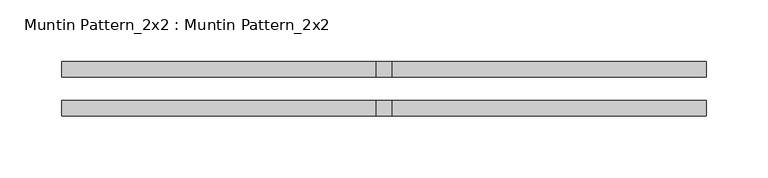
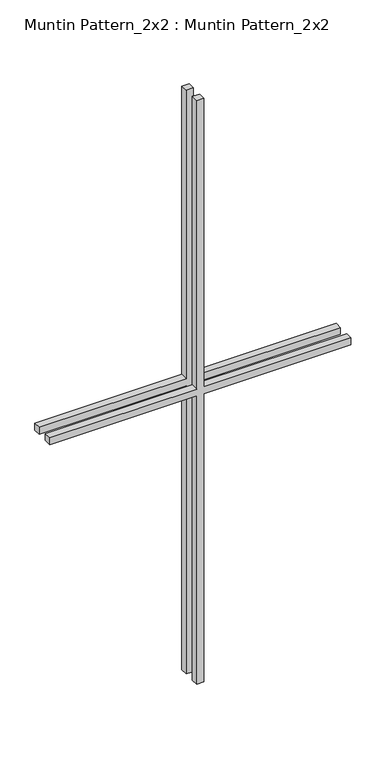
"""IFC4 building model written with IfcOpenShell, lengths in millimetres: proxy geometry, Muntin Pattern_2x2 : Muntin Pattern_2x2."""

from ifc_helpers import new_model, si_unit, frame, origin, place, context, project, spatial, polyline, outline, extrude, source, transform, mapped, element, save


def muntin_pattern_2x2_muntin_pattern_2x2_c2d27229(model_context):
    return source(origin(), model_context, "Body", "SweptSolid", [
        extrude(outline(polyline([(542.925, -6.35), (542.925, -261.9375), (530.225, -261.9375), (530.225, -6.35), (0.0, -6.35), (0.0, 6.35), (530.225, 6.35), (530.225, 261.9375), (542.925, 261.9375), (542.925, 6.35), (1073.15, 6.35), (1073.15, -6.35), (542.925, -6.35)])), frame((0.0, -22.225, 0.0), z_axis=(0.0, 1.0, 0.0), x_axis=(0.0, 0.0, 1.0)), (0.0, 0.0, 1.0), 12.7),
        extrude(outline(polyline([(542.925, -6.35), (542.925, -261.9375), (530.225, -261.9375), (530.225, -6.35), (0.0, -6.35), (0.0, 6.35), (530.225, 6.35), (530.225, 261.9375), (542.925, 261.9375), (542.925, 6.35), (1073.15, 6.35), (1073.15, -6.35), (542.925, -6.35)])), frame((0.0, 9.525, 0.0), z_axis=(0.0, 1.0, 0.0), x_axis=(0.0, 0.0, 1.0)), (0.0, 0.0, 1.0), 12.7),
    ])


if __name__ == "__main__":
    model = new_model("IFC4")
    model_context = context("Model", 3, world=origin())
    ifc_project = project(units=[si_unit("LENGTHUNIT", "METRE", prefix="MILLI")], contexts=[model_context])
    site = spatial("IfcSite", under=ifc_project)
    building = spatial("IfcBuilding", under=site)
    placement = place(None, origin())
    muntin_pattern_2x2_muntin_pattern_2x2_shape = muntin_pattern_2x2_muntin_pattern_2x2_c2d27229(model_context)
    element("IfcBuildingElementProxy", 1, Name="Muntin Pattern_2x2 : Muntin Pattern_2x2", ObjectType="Muntin Pattern_2x2 : Muntin Pattern_2x2", at=placement, inside=building, context=model_context, shape_type="MappedRepresentation", body=[
        mapped(muntin_pattern_2x2_muntin_pattern_2x2_shape, transform((0.0, 0.0, 0.0), x_axis=(1.0, 0.0, 0.0), y_axis=(0.0, 1.0, 0.0), z_axis=(0.0, 0.0, 1.0))),
    ])
    save(model, "model.ifc")

# Revit data of these elements
# Type "Muntin Pattern_2x2 : Muntin Pattern_2x2"
#   Width [instance default] = 4' - 0"
#   Thickness = 0' - 0 1/2"
#   Height [instance default] = 4' - 0"
#   Distance = 0' - 0 3/4"
#   Interior Material [instance default] = none
#   Exterior Material [instance default] = none
#   Default Elevation = 0
# Element 1 (IfcBuildingElementProxy, "Muntin Pattern_2x2 : Muntin Pattern_2x2")
#   Width = 1' - 8 5/8"
#   Height = 3' - 6 1/4"
#   Interior Material = Wood - Stained
#   Exterior Material = Clad - White
#   Materials on its faces: "Clad - White", "Wood - Stained"
# Materials
#   "Clad - White": class "Wood", colour RGB 242 242 238, transparency 0, Cost = 0
#   "Wood - Stained": class "Wood", colour RGB 224 178 126, transparency 0, Cost = 0
